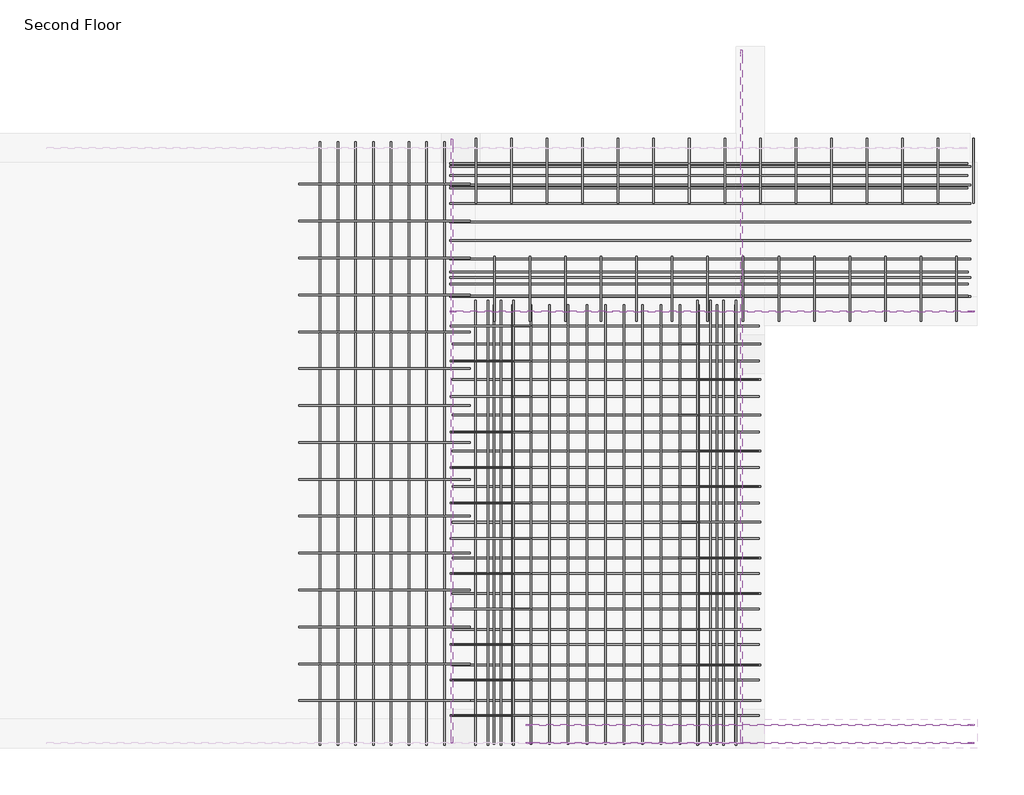
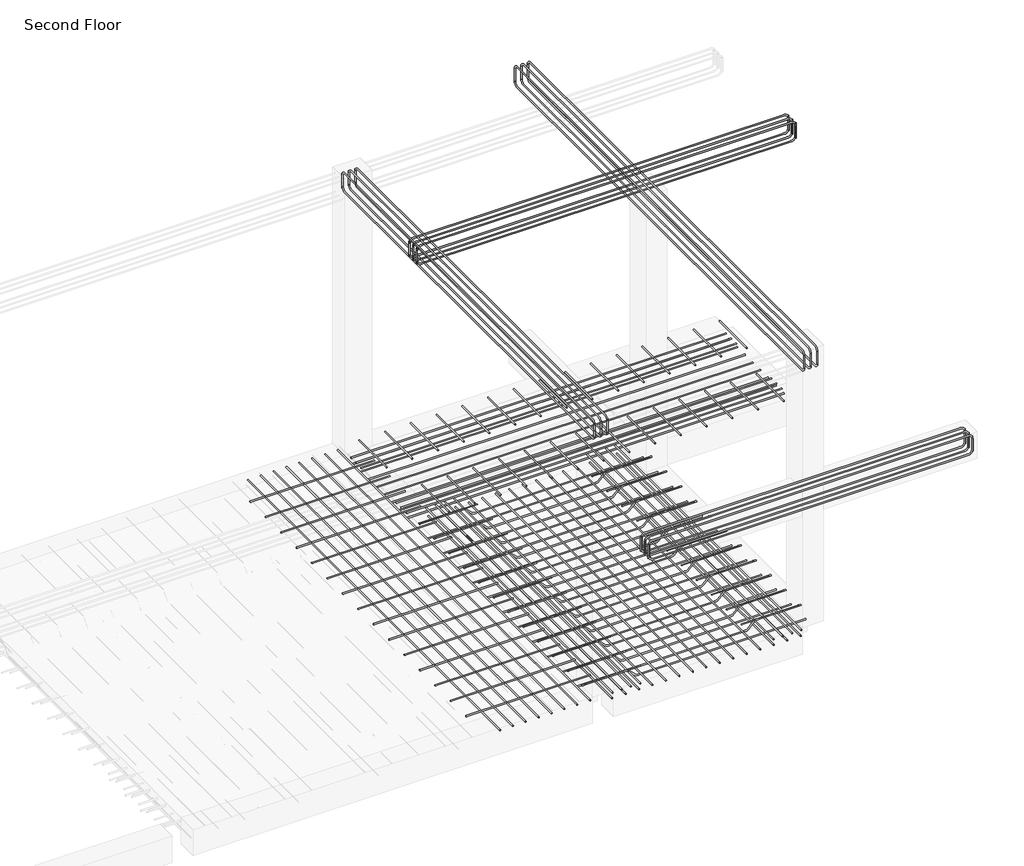
# One storey, part 4 of 4: 22 reinforcing bars.
"""IFC4 building model written with IfcOpenShell, lengths in millimetres."""

from ifc_helpers import new_model, si_unit, point, frame, origin, place, context, project, spatial, polyline, circle_curve, trimmed, segment, composite_curve, source, transform, mapped, element, save
from ifc_brep_helpers import swept_disk

model = new_model("IFC4")

# Units and contexts
model_context = context("Model", 3, world=origin())
ifc_project = project(units=[si_unit("LENGTHUNIT", "METRE", prefix="MILLI")], contexts=[model_context])

# Site, building, storey
site = spatial("IfcSite", under=ifc_project)
building = spatial("IfcBuilding", under=site)
storey = spatial("IfcBuildingStorey", under=building, Name="Second Floor", Elevation=6400.8)

# Reinforcing bars
placement = place(None, origin())
reinforcing_bar_shape = source(origin(), model_context, "Body", "SolidModel", [
    swept_disk(composite_curve([segment(polyline([(1701.2387526, 5017.2334631, 9363.3494949), (1701.2387526, 5017.2334631, 9511.3494949)]), True, "CONTINUOUS"), segment(trimmed(circle_curve(frame((1701.2387526, 4971.2334631, 9511.3494949), z_axis=(1.0, 0.0, 0.0), x_axis=(0.0, 46.0, 0.0)), 46.0), [point((1701.2387526, 5017.2334631, 9511.3494949))], [point((1701.2387526, 4971.2334631, 9557.3494949))], True, "CARTESIAN"), True, "CONTINUOUS"), segment(polyline([(1701.2387526, 4971.2334631, 9557.3494949), (1701.2387526, 278.4334631, 9557.3494949)]), True, "CONTINUOUS"), segment(trimmed(circle_curve(frame((1701.2387526, 278.4334631, 9511.3494949), z_axis=(1.0, 0.0, 0.0), x_axis=(0.0, 0.0, 46.0)), 46.0), [point((1701.2387526, 278.4334631, 9557.3494949))], [point((1701.2387526, 232.4334631, 9511.3494949))], True, "CARTESIAN"), True, "CONTINUOUS"), segment(polyline([(1701.2387526, 232.4334631, 9511.3494949), (1701.2387526, 232.4334631, 9363.3494949)]), True, "CONTINUOUS")], self_intersect=False), 6.0),
])
element("IfcReinforcingBar", 1, at=placement, inside=storey, context=model_context, shape_type="MappedRepresentation", body=[
    mapped(reinforcing_bar_shape, transform((0.0, 0.0, 0.0), x_axis=(1.0, 0.0, 0.0), y_axis=(0.0, 1.0, 0.0), z_axis=(0.0, 0.0, 1.0))),
    mapped(reinforcing_bar_shape, transform((70.4494949, 0.0, 0.0), x_axis=(1.0, 0.0, 0.0), y_axis=(0.0, 1.0, 0.0), z_axis=(0.0, 0.0, 1.0))),
    mapped(reinforcing_bar_shape, transform((140.8989899, 0.0, 0.0), x_axis=(1.0, 0.0, 0.0), y_axis=(0.0, 1.0, 0.0), z_axis=(0.0, 0.0, 1.0))),
])
reinforcing_bar_2_shape = source(origin(), model_context, "Body", "SolidModel", [
    swept_disk(composite_curve([segment(polyline([(1701.2387526, 5017.2334631, 9534.2505051), (1701.2387526, 5017.2334631, 9386.2505051)]), True, "CONTINUOUS"), segment(trimmed(circle_curve(frame((1701.2387526, 4971.2334631, 9386.2505051), z_axis=(-1.0, 0.0, 0.0), x_axis=(0.0, 46.0, 0.0)), 46.0), [point((1701.2387526, 5017.2334631, 9386.2505051))], [point((1701.2387526, 4971.2334631, 9340.2505051))], True, "CARTESIAN"), True, "CONTINUOUS"), segment(polyline([(1701.2387526, 4971.2334631, 9340.2505051), (1701.2387526, 278.4334631, 9340.2505051)]), True, "CONTINUOUS"), segment(trimmed(circle_curve(frame((1701.2387526, 278.4334631, 9386.2505051), z_axis=(-1.0, 0.0, 0.0), x_axis=(0.0, 0.0, -46.0)), 46.0), [point((1701.2387526, 278.4334631, 9340.2505051))], [point((1701.2387526, 232.4334631, 9386.2505051))], True, "CARTESIAN"), True, "CONTINUOUS"), segment(polyline([(1701.2387526, 232.4334631, 9386.2505051), (1701.2387526, 232.4334631, 9534.2505051)]), True, "CONTINUOUS")], self_intersect=False), 6.0),
])
element("IfcReinforcingBar", 2, at=placement, inside=storey, context=model_context, shape_type="MappedRepresentation", body=[
    mapped(reinforcing_bar_2_shape, transform((0.0, 0.0, 0.0), x_axis=(1.0, 0.0, 0.0), y_axis=(0.0, 1.0, 0.0), z_axis=(0.0, 0.0, 1.0))),
    mapped(reinforcing_bar_2_shape, transform((70.4494949, 0.0, 0.0), x_axis=(1.0, 0.0, 0.0), y_axis=(0.0, 1.0, 0.0), z_axis=(0.0, 0.0, 1.0))),
    mapped(reinforcing_bar_2_shape, transform((140.8989899, 0.0, 0.0), x_axis=(1.0, 0.0, 0.0), y_axis=(0.0, 1.0, 0.0), z_axis=(0.0, 0.0, 1.0))),
])
reinforcing_bar_3_shape = source(origin(), model_context, "Body", "SolidModel", [
    swept_disk(composite_curve([segment(polyline([(3999.1887526, 5724.7334631, 9364.0994949), (3999.1887526, 5724.7334631, 9512.0994949)]), True, "CONTINUOUS"), segment(trimmed(circle_curve(frame((3999.1887526, 5678.7334631, 9512.0994949), z_axis=(1.0, 0.0, 0.0), x_axis=(0.0, 46.0, 0.0)), 46.0), [point((3999.1887526, 5724.7334631, 9512.0994949))], [point((3999.1887526, 5678.7334631, 9558.0994949))], True, "CARTESIAN"), True, "CONTINUOUS"), segment(polyline([(3999.1887526, 5678.7334631, 9558.0994949), (3999.1887526, 278.4334631, 9558.0994949)]), True, "CONTINUOUS"), segment(trimmed(circle_curve(frame((3999.1887526, 278.4334631, 9512.0994949), z_axis=(1.0, 0.0, 0.0), x_axis=(0.0, 0.0, 46.0)), 46.0), [point((3999.1887526, 278.4334631, 9558.0994949))], [point((3999.1887526, 232.4334631, 9512.0994949))], True, "CARTESIAN"), True, "CONTINUOUS"), segment(polyline([(3999.1887526, 232.4334631, 9512.0994949), (3999.1887526, 232.4334631, 9364.0994949)]), True, "CONTINUOUS")], self_intersect=False), 6.0),
])
element("IfcReinforcingBar", 3, at=placement, inside=storey, context=model_context, shape_type="MappedRepresentation", body=[
    mapped(reinforcing_bar_3_shape, transform((0.0, 0.0, 0.0), x_axis=(1.0, 0.0, 0.0), y_axis=(0.0, 1.0, 0.0), z_axis=(0.0, 0.0, 1.0))),
    mapped(reinforcing_bar_3_shape, transform((71.1994949, 0.0, 0.0), x_axis=(1.0, 0.0, 0.0), y_axis=(0.0, 1.0, 0.0), z_axis=(0.0, 0.0, 1.0))),
    mapped(reinforcing_bar_3_shape, transform((142.3989899, 0.0, 0.0), x_axis=(1.0, 0.0, 0.0), y_axis=(0.0, 1.0, 0.0), z_axis=(0.0, 0.0, 1.0))),
])
reinforcing_bar_4_shape = source(origin(), model_context, "Body", "SolidModel", [
    swept_disk(composite_curve([segment(polyline([(3999.1887526, 5724.7334631, 9518.5005051), (3999.1887526, 5724.7334631, 9370.5005051)]), True, "CONTINUOUS"), segment(trimmed(circle_curve(frame((3999.1887526, 5678.7334631, 9370.5005051), z_axis=(-1.0, 0.0, 0.0), x_axis=(0.0, 46.0, 0.0)), 46.0), [point((3999.1887526, 5724.7334631, 9370.5005051))], [point((3999.1887526, 5678.7334631, 9324.5005051))], True, "CARTESIAN"), True, "CONTINUOUS"), segment(polyline([(3999.1887526, 5678.7334631, 9324.5005051), (3999.1887526, 278.4334631, 9324.5005051)]), True, "CONTINUOUS"), segment(trimmed(circle_curve(frame((3999.1887526, 278.4334631, 9370.5005051), z_axis=(-1.0, 0.0, 0.0), x_axis=(0.0, 0.0, -46.0)), 46.0), [point((3999.1887526, 278.4334631, 9324.5005051))], [point((3999.1887526, 232.4334631, 9370.5005051))], True, "CARTESIAN"), True, "CONTINUOUS"), segment(polyline([(3999.1887526, 232.4334631, 9370.5005051), (3999.1887526, 232.4334631, 9518.5005051)]), True, "CONTINUOUS")], self_intersect=False), 6.0),
])
element("IfcReinforcingBar", 4, at=placement, inside=storey, context=model_context, shape_type="MappedRepresentation", body=[
    mapped(reinforcing_bar_4_shape, transform((0.0, 0.0, 0.0), x_axis=(1.0, 0.0, 0.0), y_axis=(0.0, 1.0, 0.0), z_axis=(0.0, 0.0, 1.0))),
    mapped(reinforcing_bar_4_shape, transform((71.1994949, 0.0, 0.0), x_axis=(1.0, 0.0, 0.0), y_axis=(0.0, 1.0, 0.0), z_axis=(0.0, 0.0, 1.0))),
    mapped(reinforcing_bar_4_shape, transform((142.3989899, 0.0, 0.0), x_axis=(1.0, 0.0, 0.0), y_axis=(0.0, 1.0, 0.0), z_axis=(0.0, 0.0, 1.0))),
])
reinforcing_bar_5_shape = source(origin(), model_context, "Body", "SolidModel", [
    swept_disk(composite_curve([segment(polyline([(5841.2691711, 3584.0814555, 9362.3520076), (5841.2691711, 3584.0814555, 9510.3520076)]), True, "CONTINUOUS"), segment(trimmed(circle_curve(frame((5795.2691711, 3584.0814555, 9510.3520076), z_axis=(0.0, -1.0, 0.0), x_axis=(46.0, 0.0, 0.0)), 46.0), [point((5841.2691711, 3584.0814555, 9510.3520076))], [point((5795.2691711, 3584.0814555, 9556.3520076))], True, "CARTESIAN"), True, "CONTINUOUS"), segment(polyline([(5795.2691711, 3584.0814555, 9556.3520076), (1734.3882476, 3584.0814555, 9556.3520076)]), True, "CONTINUOUS"), segment(trimmed(circle_curve(frame((1734.3882476, 3584.0814555, 9510.3520076), z_axis=(0.0, -1.0, 0.0), x_axis=(0.0, 0.0, 46.0)), 46.0), [point((1734.3882476, 3584.0814555, 9556.3520076))], [point((1688.3882476, 3584.0814555, 9510.3520076))], True, "CARTESIAN"), True, "CONTINUOUS"), segment(polyline([(1688.3882476, 3584.0814555, 9510.3520076), (1688.3882476, 3584.0814555, 9362.3520076)]), True, "CONTINUOUS")], self_intersect=False), 6.0),
])
element("IfcReinforcingBar", 5, at=placement, inside=storey, context=model_context, shape_type="MappedRepresentation", body=[
    mapped(reinforcing_bar_5_shape, transform((0.0, 0.0, 0.0), x_axis=(1.0, 0.0, 0.0), y_axis=(0.0, 1.0, 0.0), z_axis=(0.0, 0.0, 1.0))),
    mapped(reinforcing_bar_5_shape, transform((0.0, 69.4520076, 0.0), x_axis=(1.0, 0.0, 0.0), y_axis=(0.0, 1.0, 0.0), z_axis=(0.0, 0.0, 1.0))),
    mapped(reinforcing_bar_5_shape, transform((0.0, 138.9040151, 0.0), x_axis=(1.0, 0.0, 0.0), y_axis=(0.0, 1.0, 0.0), z_axis=(0.0, 0.0, 1.0))),
])
reinforcing_bar_6_shape = source(origin(), model_context, "Body", "SolidModel", [
    swept_disk(composite_curve([segment(polyline([(5840.2625116, 3584.0814555, 9535.2479924), (5840.2625116, 3584.0814555, 9387.2479924)]), True, "CONTINUOUS"), segment(trimmed(circle_curve(frame((5794.2625116, 3584.0814555, 9387.2479924), z_axis=(0.0, 1.0, 0.0), x_axis=(46.0, 0.0, 0.0)), 46.0), [point((5840.2625116, 3584.0814555, 9387.2479924))], [point((5794.2625116, 3584.0814555, 9341.2479924))], True, "CARTESIAN"), True, "CONTINUOUS"), segment(polyline([(5794.2625116, 3584.0814555, 9341.2479924), (1734.3882476, 3584.0814555, 9341.2479924)]), True, "CONTINUOUS"), segment(trimmed(circle_curve(frame((1734.3882476, 3584.0814555, 9387.2479924), z_axis=(0.0, 1.0, 0.0), x_axis=(0.0, 0.0, -46.0)), 46.0), [point((1734.3882476, 3584.0814555, 9341.2479924))], [point((1688.3882476, 3584.0814555, 9387.2479924))], True, "CARTESIAN"), True, "CONTINUOUS"), segment(polyline([(1688.3882476, 3584.0814555, 9387.2479924), (1688.3882476, 3584.0814555, 9535.2479924)]), True, "CONTINUOUS")], self_intersect=False), 6.0),
])
element("IfcReinforcingBar", 6, at=placement, inside=storey, context=model_context, shape_type="MappedRepresentation", body=[
    mapped(reinforcing_bar_6_shape, transform((0.0, 0.0, 0.0), x_axis=(1.0, 0.0, 0.0), y_axis=(0.0, 1.0, 0.0), z_axis=(0.0, 0.0, 1.0))),
    mapped(reinforcing_bar_6_shape, transform((0.0, 69.4520076, 0.0), x_axis=(1.0, 0.0, 0.0), y_axis=(0.0, 1.0, 0.0), z_axis=(0.0, 0.0, 1.0))),
    mapped(reinforcing_bar_6_shape, transform((0.0, 138.9040151, 0.0), x_axis=(1.0, 0.0, 0.0), y_axis=(0.0, 1.0, 0.0), z_axis=(0.0, 0.0, 1.0))),
])
reinforcing_bar_7_shape = source(origin(), model_context, "Body", "SolidModel", [
    swept_disk(composite_curve([segment(polyline([(5841.2691711, 229.5339681, 7763.8994949), (5841.2691711, 229.5339681, 7911.8994949)]), True, "CONTINUOUS"), segment(trimmed(circle_curve(frame((5795.2691711, 229.5339681, 7911.8994949), z_axis=(0.0, -1.0, 0.0), x_axis=(46.0, 0.0, 0.0)), 46.0), [point((5841.2691711, 229.5339681, 7911.8994949))], [point((5795.2691711, 229.5339681, 7957.8994949))], True, "CARTESIAN"), True, "CONTINUOUS"), segment(polyline([(5795.2691711, 229.5339681, 7957.8994949), (2337.5636354, 229.5339681, 7957.8994949)]), True, "CONTINUOUS"), segment(trimmed(circle_curve(frame((2337.5636354, 229.5339681, 7911.8994949), z_axis=(0.0, -1.0, 0.0), x_axis=(0.0, 0.0, 46.0)), 46.0), [point((2337.5636354, 229.5339681, 7957.8994949))], [point((2291.5636354, 229.5339681, 7911.8994949))], True, "CARTESIAN"), True, "CONTINUOUS"), segment(polyline([(2291.5636354, 229.5339681, 7911.8994949), (2291.5636354, 229.5339681, 7763.8994949)]), True, "CONTINUOUS")], self_intersect=False), 6.0),
])
element("IfcReinforcingBar", 7, at=placement, inside=storey, context=model_context, shape_type="MappedRepresentation", body=[
    mapped(reinforcing_bar_7_shape, transform((0.0, 0.0, 0.0), x_axis=(1.0, 0.0, 0.0), y_axis=(0.0, 1.0, 0.0), z_axis=(0.0, 0.0, 1.0))),
    mapped(reinforcing_bar_7_shape, transform((0.0, 71.1994949, 0.0), x_axis=(1.0, 0.0, 0.0), y_axis=(0.0, 1.0, 0.0), z_axis=(0.0, 0.0, 1.0))),
    mapped(reinforcing_bar_7_shape, transform((0.0, 142.3989899, 0.0), x_axis=(1.0, 0.0, 0.0), y_axis=(0.0, 1.0, 0.0), z_axis=(0.0, 0.0, 1.0))),
])
reinforcing_bar_8_shape = source(origin(), model_context, "Body", "SolidModel", [
    swept_disk(composite_curve([segment(polyline([(5840.2625116, 229.5339681, 7933.3005051), (5840.2625116, 229.5339681, 7785.3005051)]), True, "CONTINUOUS"), segment(trimmed(circle_curve(frame((5794.2625116, 229.5339681, 7785.3005051), z_axis=(0.0, 1.0, 0.0), x_axis=(46.0, 0.0, 0.0)), 46.0), [point((5840.2625116, 229.5339681, 7785.3005051))], [point((5794.2625116, 229.5339681, 7739.3005051))], True, "CARTESIAN"), True, "CONTINUOUS"), segment(polyline([(5794.2625116, 229.5339681, 7739.3005051), (2341.190873, 229.5339681, 7739.3005051)]), True, "CONTINUOUS"), segment(trimmed(circle_curve(frame((2341.190873, 229.5339681, 7785.3005051), z_axis=(0.0, 1.0, 0.0), x_axis=(0.0, 0.0, -46.0)), 46.0), [point((2341.190873, 229.5339681, 7739.3005051))], [point((2295.190873, 229.5339681, 7785.3005051))], True, "CARTESIAN"), True, "CONTINUOUS"), segment(polyline([(2295.190873, 229.5339681, 7785.3005051), (2295.190873, 229.5339681, 7933.3005051)]), True, "CONTINUOUS")], self_intersect=False), 6.0),
])
element("IfcReinforcingBar", 8, at=placement, inside=storey, context=model_context, shape_type="MappedRepresentation", body=[
    mapped(reinforcing_bar_8_shape, transform((0.0, 0.0, 0.0), x_axis=(1.0, 0.0, 0.0), y_axis=(0.0, 1.0, 0.0), z_axis=(0.0, 0.0, 1.0))),
    mapped(reinforcing_bar_8_shape, transform((0.0, 71.1994949, 0.0), x_axis=(1.0, 0.0, 0.0), y_axis=(0.0, 1.0, 0.0), z_axis=(0.0, 0.0, 1.0))),
    mapped(reinforcing_bar_8_shape, transform((0.0, 142.3989899, 0.0), x_axis=(1.0, 0.0, 0.0), y_axis=(0.0, 1.0, 0.0), z_axis=(0.0, 0.0, 1.0))),
])
reinforcing_bar_9_shape = source(origin(), model_context, "Body", "SolidModel", [
    swept_disk(composite_curve([segment(polyline([(1688.7874305, 3539.2334631, 6369.8), (2168.5956769, 3539.2334631, 6369.8)]), True, "CONTINUOUS"), segment(trimmed(circle_curve(frame((2168.5956769, 3539.2334631, 6323.8), z_axis=(0.0, 1.0, 0.0), x_axis=(0.0, 0.0, 46.0)), 46.0), [point((2168.5956769, 3539.2334631, 6369.8))], [point((2201.1225888, 3539.2334631, 6356.3269119))], True, "CARTESIAN"), True, "CONTINUOUS"), segment(polyline([(2201.1225888, 3539.2334631, 6356.3269119), (2264.5764127, 3539.2334631, 6292.8730881)]), True, "CONTINUOUS"), segment(trimmed(circle_curve(frame((2297.1033246, 3539.2334631, 6325.4), z_axis=(0.0, -1.0, 0.0), x_axis=(-32.52691189999996, 0.0, -32.526911899999504)), 46.0), [point((2264.5764127, 3539.2334631, 6292.8730881))], [point((2297.1033246, 3539.2334631, 6279.4))], True, "CARTESIAN"), True, "CONTINUOUS"), segment(polyline([(2297.1033246, 3539.2334631, 6279.4), (4139.8402551, 3539.2334631, 6279.4)]), True, "CONTINUOUS")], self_intersect=False), 6.0),
])
element("IfcReinforcingBar", 9, at=placement, inside=storey, context=model_context, shape_type="MappedRepresentation", body=[
    mapped(reinforcing_bar_9_shape, transform((0.0, 0.0, 0.0), x_axis=(1.0, 0.0, 0.0), y_axis=(0.0, 1.0, 0.0), z_axis=(0.0, 0.0, 1.0))),
    mapped(reinforcing_bar_9_shape, transform((0.0, -281.0909091, 0.0), x_axis=(1.0, 0.0, 0.0), y_axis=(0.0, 1.0, 0.0), z_axis=(0.0, 0.0, 1.0))),
    mapped(reinforcing_bar_9_shape, transform((0.0, -562.1818182, 0.0), x_axis=(1.0, 0.0, 0.0), y_axis=(0.0, 1.0, 0.0), z_axis=(0.0, 0.0, 1.0))),
    mapped(reinforcing_bar_9_shape, transform((0.0, -843.2727273, 0.0), x_axis=(1.0, 0.0, 0.0), y_axis=(0.0, 1.0, 0.0), z_axis=(0.0, 0.0, 1.0))),
    mapped(reinforcing_bar_9_shape, transform((0.0, -1124.3636364, 0.0), x_axis=(1.0, 0.0, 0.0), y_axis=(0.0, 1.0, 0.0), z_axis=(0.0, 0.0, 1.0))),
    mapped(reinforcing_bar_9_shape, transform((0.0, -1405.4545455, 0.0), x_axis=(1.0, 0.0, 0.0), y_axis=(0.0, 1.0, 0.0), z_axis=(0.0, 0.0, 1.0))),
    mapped(reinforcing_bar_9_shape, transform((0.0, -1686.5454545, 0.0), x_axis=(1.0, 0.0, 0.0), y_axis=(0.0, 1.0, 0.0), z_axis=(0.0, 0.0, 1.0))),
    mapped(reinforcing_bar_9_shape, transform((0.0, -1967.6363636, 0.0), x_axis=(1.0, 0.0, 0.0), y_axis=(0.0, 1.0, 0.0), z_axis=(0.0, 0.0, 1.0))),
    mapped(reinforcing_bar_9_shape, transform((0.0, -2248.7272727, 0.0), x_axis=(1.0, 0.0, 0.0), y_axis=(0.0, 1.0, 0.0), z_axis=(0.0, 0.0, 1.0))),
    mapped(reinforcing_bar_9_shape, transform((0.0, -2529.8181818, 0.0), x_axis=(1.0, 0.0, 0.0), y_axis=(0.0, 1.0, 0.0), z_axis=(0.0, 0.0, 1.0))),
    mapped(reinforcing_bar_9_shape, transform((0.0, -2810.9090909, 0.0), x_axis=(1.0, 0.0, 0.0), y_axis=(0.0, 1.0, 0.0), z_axis=(0.0, 0.0, 1.0))),
    mapped(reinforcing_bar_9_shape, transform((0.0, -3092.0, 0.0), x_axis=(1.0, 0.0, 0.0), y_axis=(0.0, 1.0, 0.0), z_axis=(0.0, 0.0, 1.0))),
])
reinforcing_bar_10_shape = source(origin(), model_context, "Body", "SolidModel", [
    swept_disk(composite_curve([segment(polyline([(4153.2890646, 564.2307141, 6369.8), (3672.2951557, 564.2307141, 6369.8)]), True, "CONTINUOUS"), segment(trimmed(circle_curve(frame((3672.2951557, 564.2307141, 6323.8), z_axis=(0.0, -1.0, 0.0), x_axis=(0.0, 0.0, 46.0)), 46.0), [point((3672.2951557, 564.2307141, 6369.8))], [point((3639.7682438, 564.2307141, 6356.3269119))], True, "CARTESIAN"), True, "CONTINUOUS"), segment(polyline([(3639.7682438, 564.2307141, 6356.3269119), (3576.3144199, 564.2307141, 6292.8730881)]), True, "CONTINUOUS"), segment(trimmed(circle_curve(frame((3543.787508, 564.2307141, 6325.4), z_axis=(0.0, 1.0000000000000002, 0.0), x_axis=(32.52691189999996, 0.0, -32.526911899999504)), 46.0), [point((3576.3144199, 564.2307141, 6292.8730881))], [point((3543.787508, 564.2307141, 6279.4))], True, "CARTESIAN"), True, "CONTINUOUS"), segment(polyline([(3543.787508, 564.2307141, 6279.4), (1702.23624, 564.2307141, 6279.4)]), True, "CONTINUOUS")], self_intersect=False), 6.0),
])
element("IfcReinforcingBar", 10, at=placement, inside=storey, context=model_context, shape_type="MappedRepresentation", body=[
    mapped(reinforcing_bar_10_shape, transform((0.0, 0.0, 0.0), x_axis=(1.0, 0.0, 0.0), y_axis=(0.0, 1.0, 0.0), z_axis=(0.0, 0.0, 1.0))),
    mapped(reinforcing_bar_10_shape, transform((0.0, 283.1945647, 0.0), x_axis=(1.0, 0.0, 0.0), y_axis=(0.0, 1.0, 0.0), z_axis=(0.0, 0.0, 1.0))),
    mapped(reinforcing_bar_10_shape, transform((0.0, 566.3891295, 0.0), x_axis=(1.0, 0.0, 0.0), y_axis=(0.0, 1.0, 0.0), z_axis=(0.0, 0.0, 1.0))),
    mapped(reinforcing_bar_10_shape, transform((0.0, 849.5836942, 0.0), x_axis=(1.0, 0.0, 0.0), y_axis=(0.0, 1.0, 0.0), z_axis=(0.0, 0.0, 1.0))),
    mapped(reinforcing_bar_10_shape, transform((0.0, 1132.778259, 0.0), x_axis=(1.0, 0.0, 0.0), y_axis=(0.0, 1.0, 0.0), z_axis=(0.0, 0.0, 1.0))),
    mapped(reinforcing_bar_10_shape, transform((0.0, 1415.9728237, 0.0), x_axis=(1.0, 0.0, 0.0), y_axis=(0.0, 1.0, 0.0), z_axis=(0.0, 0.0, 1.0))),
    mapped(reinforcing_bar_10_shape, transform((0.0, 1699.1673885, 0.0), x_axis=(1.0, 0.0, 0.0), y_axis=(0.0, 1.0, 0.0), z_axis=(0.0, 0.0, 1.0))),
    mapped(reinforcing_bar_10_shape, transform((0.0, 1982.3619532, 0.0), x_axis=(1.0, 0.0, 0.0), y_axis=(0.0, 1.0, 0.0), z_axis=(0.0, 0.0, 1.0))),
    mapped(reinforcing_bar_10_shape, transform((0.0, 2265.556518, 0.0), x_axis=(1.0, 0.0, 0.0), y_axis=(0.0, 1.0, 0.0), z_axis=(0.0, 0.0, 1.0))),
    mapped(reinforcing_bar_10_shape, transform((0.0, 2548.7510827, 0.0), x_axis=(1.0, 0.0, 0.0), y_axis=(0.0, 1.0, 0.0), z_axis=(0.0, 0.0, 1.0))),
    mapped(reinforcing_bar_10_shape, transform((0.0, 2831.9456475, 0.0), x_axis=(1.0, 0.0, 0.0), y_axis=(0.0, 1.0, 0.0), z_axis=(0.0, 0.0, 1.0))),
])
reinforcing_bar_11_shape = source(origin(), model_context, "Body", "SolidModel", [
    swept_disk(composite_curve([segment(polyline([(3650.7560505, 3742.8334631, 6359.5006995), (3650.7560505, 211.4334631, 6359.5006995)]), True, "CONTINUOUS")], self_intersect=False), 6.0),
])
element("IfcReinforcingBar", 11, at=placement, inside=storey, context=model_context, shape_type="MappedRepresentation", body=[
    mapped(reinforcing_bar_11_shape, transform((0.0, 0.0, 0.0), x_axis=(1.0, 0.0, 0.0), y_axis=(0.0, 1.0, 0.0), z_axis=(0.0, 0.0, 1.0))),
    mapped(reinforcing_bar_11_shape, transform((101.777399, 0.0, 0.0), x_axis=(1.0, 0.0, 0.0), y_axis=(0.0, 1.0, 0.0), z_axis=(0.0, 0.0, 1.0))),
    mapped(reinforcing_bar_11_shape, transform((203.554798, 0.0, 0.0), x_axis=(1.0, 0.0, 0.0), y_axis=(0.0, 1.0, 0.0), z_axis=(0.0, 0.0, 1.0))),
    mapped(reinforcing_bar_11_shape, transform((305.3321971, 0.0, 0.0), x_axis=(1.0, 0.0, 0.0), y_axis=(0.0, 1.0, 0.0), z_axis=(0.0, 0.0, 1.0))),
])
reinforcing_bar_12_shape = source(origin(), model_context, "Body", "SolidModel", [
    swept_disk(composite_curve([segment(polyline([(1697.8477074, 3539.2334631, 6371.8), (2325.3671503, 3539.2334631, 6371.8)]), True, "CONTINUOUS")], self_intersect=False), 4.0),
])
element("IfcReinforcingBar", 12, at=placement, inside=storey, context=model_context, shape_type="MappedRepresentation", body=[
    mapped(reinforcing_bar_12_shape, transform((0.0, 0.0, 0.0), x_axis=(1.0, 0.0, 0.0), y_axis=(0.0, 1.0, 0.0), z_axis=(0.0, 0.0, 1.0))),
    mapped(reinforcing_bar_12_shape, transform((0.0, -281.0909091, 0.0), x_axis=(1.0, 0.0, 0.0), y_axis=(0.0, 1.0, 0.0), z_axis=(0.0, 0.0, 1.0))),
    mapped(reinforcing_bar_12_shape, transform((0.0, -562.1818182, 0.0), x_axis=(1.0, 0.0, 0.0), y_axis=(0.0, 1.0, 0.0), z_axis=(0.0, 0.0, 1.0))),
    mapped(reinforcing_bar_12_shape, transform((0.0, -843.2727273, 0.0), x_axis=(1.0, 0.0, 0.0), y_axis=(0.0, 1.0, 0.0), z_axis=(0.0, 0.0, 1.0))),
    mapped(reinforcing_bar_12_shape, transform((0.0, -1124.3636364, 0.0), x_axis=(1.0, 0.0, 0.0), y_axis=(0.0, 1.0, 0.0), z_axis=(0.0, 0.0, 1.0))),
    mapped(reinforcing_bar_12_shape, transform((0.0, -1405.4545455, 0.0), x_axis=(1.0, 0.0, 0.0), y_axis=(0.0, 1.0, 0.0), z_axis=(0.0, 0.0, 1.0))),
    mapped(reinforcing_bar_12_shape, transform((0.0, -1686.5454545, 0.0), x_axis=(1.0, 0.0, 0.0), y_axis=(0.0, 1.0, 0.0), z_axis=(0.0, 0.0, 1.0))),
    mapped(reinforcing_bar_12_shape, transform((0.0, -1967.6363636, 0.0), x_axis=(1.0, 0.0, 0.0), y_axis=(0.0, 1.0, 0.0), z_axis=(0.0, 0.0, 1.0))),
    mapped(reinforcing_bar_12_shape, transform((0.0, -2248.7272727, 0.0), x_axis=(1.0, 0.0, 0.0), y_axis=(0.0, 1.0, 0.0), z_axis=(0.0, 0.0, 1.0))),
    mapped(reinforcing_bar_12_shape, transform((0.0, -2529.8181818, 0.0), x_axis=(1.0, 0.0, 0.0), y_axis=(0.0, 1.0, 0.0), z_axis=(0.0, 0.0, 1.0))),
    mapped(reinforcing_bar_12_shape, transform((0.0, -2810.9090909, 0.0), x_axis=(1.0, 0.0, 0.0), y_axis=(0.0, 1.0, 0.0), z_axis=(0.0, 0.0, 1.0))),
    mapped(reinforcing_bar_12_shape, transform((0.0, -3092.0, 0.0), x_axis=(1.0, 0.0, 0.0), y_axis=(0.0, 1.0, 0.0), z_axis=(0.0, 0.0, 1.0))),
])
reinforcing_bar_13_shape = source(origin(), model_context, "Body", "SolidModel", [
    swept_disk(composite_curve([segment(polyline([(4130.5876361, 3396.1763616, 6371.8), (3500.3340616, 3396.1763616, 6371.8)]), True, "CONTINUOUS")], self_intersect=False), 4.0),
])
element("IfcReinforcingBar", 13, at=placement, inside=storey, context=model_context, shape_type="MappedRepresentation", body=[
    mapped(reinforcing_bar_13_shape, transform((0.0, 0.0, 0.0), x_axis=(1.0, 0.0, 0.0), y_axis=(0.0, 1.0, 0.0), z_axis=(0.0, 0.0, 1.0))),
    mapped(reinforcing_bar_13_shape, transform((0.0, -283.1945647, 0.0), x_axis=(1.0, 0.0, 0.0), y_axis=(0.0, 1.0, 0.0), z_axis=(0.0, 0.0, 1.0))),
    mapped(reinforcing_bar_13_shape, transform((0.0, -566.3891295, 0.0), x_axis=(1.0, 0.0, 0.0), y_axis=(0.0, 1.0, 0.0), z_axis=(0.0, 0.0, 1.0))),
    mapped(reinforcing_bar_13_shape, transform((0.0, -849.5836942, 0.0), x_axis=(1.0, 0.0, 0.0), y_axis=(0.0, 1.0, 0.0), z_axis=(0.0, 0.0, 1.0))),
    mapped(reinforcing_bar_13_shape, transform((0.0, -1132.778259, 0.0), x_axis=(1.0, 0.0, 0.0), y_axis=(0.0, 1.0, 0.0), z_axis=(0.0, 0.0, 1.0))),
    mapped(reinforcing_bar_13_shape, transform((0.0, -1415.9728237, 0.0), x_axis=(1.0, 0.0, 0.0), y_axis=(0.0, 1.0, 0.0), z_axis=(0.0, 0.0, 1.0))),
    mapped(reinforcing_bar_13_shape, transform((0.0, -1699.1673885, 0.0), x_axis=(1.0, 0.0, 0.0), y_axis=(0.0, 1.0, 0.0), z_axis=(0.0, 0.0, 1.0))),
    mapped(reinforcing_bar_13_shape, transform((0.0, -1982.3619532, 0.0), x_axis=(1.0, 0.0, 0.0), y_axis=(0.0, 1.0, 0.0), z_axis=(0.0, 0.0, 1.0))),
    mapped(reinforcing_bar_13_shape, transform((0.0, -2265.556518, 0.0), x_axis=(1.0, 0.0, 0.0), y_axis=(0.0, 1.0, 0.0), z_axis=(0.0, 0.0, 1.0))),
    mapped(reinforcing_bar_13_shape, transform((0.0, -2548.7510827, 0.0), x_axis=(1.0, 0.0, 0.0), y_axis=(0.0, 1.0, 0.0), z_axis=(0.0, 0.0, 1.0))),
    mapped(reinforcing_bar_13_shape, transform((0.0, -2831.9456475, 0.0), x_axis=(1.0, 0.0, 0.0), y_axis=(0.0, 1.0, 0.0), z_axis=(0.0, 0.0, 1.0))),
])
reinforcing_bar_14_shape = source(origin(), model_context, "Body", "SolidModel", [
    swept_disk(composite_curve([segment(polyline([(3952.0882476, 218.9117605, 6287.9387401), (3952.0882476, 3706.6679133, 6287.9387401)]), True, "CONTINUOUS")], self_intersect=False), 6.0),
])
element("IfcReinforcingBar", 14, at=placement, inside=storey, context=model_context, shape_type="MappedRepresentation", body=[
    mapped(reinforcing_bar_14_shape, transform((0.0, 0.0, 0.0), x_axis=(1.0, 0.0, 0.0), y_axis=(0.0, 1.0, 0.0), z_axis=(0.0, 0.0, 1.0))),
    mapped(reinforcing_bar_14_shape, transform((-147.5785714, 0.0, 0.0), x_axis=(1.0, 0.0, 0.0), y_axis=(0.0, 1.0, 0.0), z_axis=(0.0, 0.0, 1.0))),
    mapped(reinforcing_bar_14_shape, transform((-295.1571429, 0.0, 0.0), x_axis=(1.0, 0.0, 0.0), y_axis=(0.0, 1.0, 0.0), z_axis=(0.0, 0.0, 1.0))),
    mapped(reinforcing_bar_14_shape, transform((-442.7357143, 0.0, 0.0), x_axis=(1.0, 0.0, 0.0), y_axis=(0.0, 1.0, 0.0), z_axis=(0.0, 0.0, 1.0))),
    mapped(reinforcing_bar_14_shape, transform((-590.3142857, 0.0, 0.0), x_axis=(1.0, 0.0, 0.0), y_axis=(0.0, 1.0, 0.0), z_axis=(0.0, 0.0, 1.0))),
    mapped(reinforcing_bar_14_shape, transform((-737.8928571, 0.0, 0.0), x_axis=(1.0, 0.0, 0.0), y_axis=(0.0, 1.0, 0.0), z_axis=(0.0, 0.0, 1.0))),
    mapped(reinforcing_bar_14_shape, transform((-885.4714286, 0.0, 0.0), x_axis=(1.0, 0.0, 0.0), y_axis=(0.0, 1.0, 0.0), z_axis=(0.0, 0.0, 1.0))),
    mapped(reinforcing_bar_14_shape, transform((-1033.05, 0.0, 0.0), x_axis=(1.0, 0.0, 0.0), y_axis=(0.0, 1.0, 0.0), z_axis=(0.0, 0.0, 1.0))),
    mapped(reinforcing_bar_14_shape, transform((-1180.6285714, 0.0, 0.0), x_axis=(1.0, 0.0, 0.0), y_axis=(0.0, 1.0, 0.0), z_axis=(0.0, 0.0, 1.0))),
    mapped(reinforcing_bar_14_shape, transform((-1328.2071429, 0.0, 0.0), x_axis=(1.0, 0.0, 0.0), y_axis=(0.0, 1.0, 0.0), z_axis=(0.0, 0.0, 1.0))),
    mapped(reinforcing_bar_14_shape, transform((-1475.7857143, 0.0, 0.0), x_axis=(1.0, 0.0, 0.0), y_axis=(0.0, 1.0, 0.0), z_axis=(0.0, 0.0, 1.0))),
    mapped(reinforcing_bar_14_shape, transform((-1623.3642857, 0.0, 0.0), x_axis=(1.0, 0.0, 0.0), y_axis=(0.0, 1.0, 0.0), z_axis=(0.0, 0.0, 1.0))),
    mapped(reinforcing_bar_14_shape, transform((-1770.9428571, 0.0, 0.0), x_axis=(1.0, 0.0, 0.0), y_axis=(0.0, 1.0, 0.0), z_axis=(0.0, 0.0, 1.0))),
    mapped(reinforcing_bar_14_shape, transform((-1918.5214286, 0.0, 0.0), x_axis=(1.0, 0.0, 0.0), y_axis=(0.0, 1.0, 0.0), z_axis=(0.0, 0.0, 1.0))),
    mapped(reinforcing_bar_14_shape, transform((-2066.1, 0.0, 0.0), x_axis=(1.0, 0.0, 0.0), y_axis=(0.0, 1.0, 0.0), z_axis=(0.0, 0.0, 1.0))),
])
reinforcing_bar_15_shape = source(origin(), model_context, "Body", "SolidModel", [
    swept_disk(composite_curve([segment(polyline([(2190.1347821, 3742.8334631, 6359.5006995), (2190.1347821, 211.4334631, 6359.5006995)]), True, "CONTINUOUS")], self_intersect=False), 6.0),
])
element("IfcReinforcingBar", 15, at=placement, inside=storey, context=model_context, shape_type="MappedRepresentation", body=[
    mapped(reinforcing_bar_15_shape, transform((0.0, 0.0, 0.0), x_axis=(1.0, 0.0, 0.0), y_axis=(0.0, 1.0, 0.0), z_axis=(0.0, 0.0, 1.0))),
    mapped(reinforcing_bar_15_shape, transform((-101.3821782, 0.0, 0.0), x_axis=(1.0, 0.0, 0.0), y_axis=(0.0, 1.0, 0.0), z_axis=(0.0, 0.0, 1.0))),
    mapped(reinforcing_bar_15_shape, transform((-202.7643564, 0.0, 0.0), x_axis=(1.0, 0.0, 0.0), y_axis=(0.0, 1.0, 0.0), z_axis=(0.0, 0.0, 1.0))),
    mapped(reinforcing_bar_15_shape, transform((-304.1465345, 0.0, 0.0), x_axis=(1.0, 0.0, 0.0), y_axis=(0.0, 1.0, 0.0), z_axis=(0.0, 0.0, 1.0))),
])
reinforcing_bar_16_shape = source(origin(), model_context, "Body", "SolidModel", [
    swept_disk(composite_curve([segment(polyline([(654.4332967, 4999.0798317, 6354.8697281), (654.4332967, 211.4334631, 6354.8697281)]), True, "CONTINUOUS")], self_intersect=False), 6.0),
])
element("IfcReinforcingBar", 16, at=placement, inside=storey, context=model_context, shape_type="MappedRepresentation", body=[
    mapped(reinforcing_bar_16_shape, transform((0.0, 0.0, 0.0), x_axis=(1.0, 0.0, 0.0), y_axis=(0.0, 1.0, 0.0), z_axis=(0.0, 0.0, 1.0))),
    mapped(reinforcing_bar_16_shape, transform((140.8412233, 0.0, 0.0), x_axis=(1.0, 0.0, 0.0), y_axis=(0.0, 1.0, 0.0), z_axis=(0.0, 0.0, 1.0))),
    mapped(reinforcing_bar_16_shape, transform((281.6824466, 0.0, 0.0), x_axis=(1.0, 0.0, 0.0), y_axis=(0.0, 1.0, 0.0), z_axis=(0.0, 0.0, 1.0))),
    mapped(reinforcing_bar_16_shape, transform((422.5236699, 0.0, 0.0), x_axis=(1.0, 0.0, 0.0), y_axis=(0.0, 1.0, 0.0), z_axis=(0.0, 0.0, 1.0))),
    mapped(reinforcing_bar_16_shape, transform((563.3648932, 0.0, 0.0), x_axis=(1.0, 0.0, 0.0), y_axis=(0.0, 1.0, 0.0), z_axis=(0.0, 0.0, 1.0))),
    mapped(reinforcing_bar_16_shape, transform((704.2061164, 0.0, 0.0), x_axis=(1.0, 0.0, 0.0), y_axis=(0.0, 1.0, 0.0), z_axis=(0.0, 0.0, 1.0))),
    mapped(reinforcing_bar_16_shape, transform((845.0473397, 0.0, 0.0), x_axis=(1.0, 0.0, 0.0), y_axis=(0.0, 1.0, 0.0), z_axis=(0.0, 0.0, 1.0))),
    mapped(reinforcing_bar_16_shape, transform((985.888563, 0.0, 0.0), x_axis=(1.0, 0.0, 0.0), y_axis=(0.0, 1.0, 0.0), z_axis=(0.0, 0.0, 1.0))),
])
reinforcing_bar_17_shape = source(origin(), model_context, "Body", "SolidModel", [
    swept_disk(composite_curve([segment(polyline([(1844.9074635, 564.2307141, 6364.2017937), (483.2910842, 564.2307141, 6364.2017937)]), True, "CONTINUOUS")], self_intersect=False), 6.0),
])
element("IfcReinforcingBar", 17, at=placement, inside=storey, context=model_context, shape_type="MappedRepresentation", body=[
    mapped(reinforcing_bar_17_shape, transform((0.0, 0.0, 0.0), x_axis=(1.0, 0.0, 0.0), y_axis=(0.0, 1.0, 0.0), z_axis=(0.0, 0.0, 1.0))),
    mapped(reinforcing_bar_17_shape, transform((0.0, 292.7783831, 0.0), x_axis=(1.0, 0.0, 0.0), y_axis=(0.0, 1.0, 0.0), z_axis=(0.0, 0.0, 1.0))),
    mapped(reinforcing_bar_17_shape, transform((0.0, 585.5567661, 0.0), x_axis=(1.0, 0.0, 0.0), y_axis=(0.0, 1.0, 0.0), z_axis=(0.0, 0.0, 1.0))),
    mapped(reinforcing_bar_17_shape, transform((0.0, 878.3351492, 0.0), x_axis=(1.0, 0.0, 0.0), y_axis=(0.0, 1.0, 0.0), z_axis=(0.0, 0.0, 1.0))),
    mapped(reinforcing_bar_17_shape, transform((0.0, 1171.1135323, 0.0), x_axis=(1.0, 0.0, 0.0), y_axis=(0.0, 1.0, 0.0), z_axis=(0.0, 0.0, 1.0))),
    mapped(reinforcing_bar_17_shape, transform((0.0, 1463.8919154, 0.0), x_axis=(1.0, 0.0, 0.0), y_axis=(0.0, 1.0, 0.0), z_axis=(0.0, 0.0, 1.0))),
    mapped(reinforcing_bar_17_shape, transform((0.0, 1756.6702984, 0.0), x_axis=(1.0, 0.0, 0.0), y_axis=(0.0, 1.0, 0.0), z_axis=(0.0, 0.0, 1.0))),
    mapped(reinforcing_bar_17_shape, transform((0.0, 2049.4486815, 0.0), x_axis=(1.0, 0.0, 0.0), y_axis=(0.0, 1.0, 0.0), z_axis=(0.0, 0.0, 1.0))),
    mapped(reinforcing_bar_17_shape, transform((0.0, 2342.2270646, 0.0), x_axis=(1.0, 0.0, 0.0), y_axis=(0.0, 1.0, 0.0), z_axis=(0.0, 0.0, 1.0))),
    mapped(reinforcing_bar_17_shape, transform((0.0, 2635.0054477, 0.0), x_axis=(1.0, 0.0, 0.0), y_axis=(0.0, 1.0, 0.0), z_axis=(0.0, 0.0, 1.0))),
    mapped(reinforcing_bar_17_shape, transform((0.0, 2927.7838307, 0.0), x_axis=(1.0, 0.0, 0.0), y_axis=(0.0, 1.0, 0.0), z_axis=(0.0, 0.0, 1.0))),
    mapped(reinforcing_bar_17_shape, transform((0.0, 3220.5622138, 0.0), x_axis=(1.0, 0.0, 0.0), y_axis=(0.0, 1.0, 0.0), z_axis=(0.0, 0.0, 1.0))),
    mapped(reinforcing_bar_17_shape, transform((0.0, 3513.3405969, 0.0), x_axis=(1.0, 0.0, 0.0), y_axis=(0.0, 1.0, 0.0), z_axis=(0.0, 0.0, 1.0))),
    mapped(reinforcing_bar_17_shape, transform((0.0, 3806.11898, 0.0), x_axis=(1.0, 0.0, 0.0), y_axis=(0.0, 1.0, 0.0), z_axis=(0.0, 0.0, 1.0))),
    mapped(reinforcing_bar_17_shape, transform((0.0, 4098.897363, 0.0), x_axis=(1.0, 0.0, 0.0), y_axis=(0.0, 1.0, 0.0), z_axis=(0.0, 0.0, 1.0))),
])
reinforcing_bar_18_shape = source(origin(), model_context, "Body", "SolidModel", [
    swept_disk(composite_curve([segment(polyline([(5796.3354159, 4634.2611065, 6354.7212824), (1682.3882476, 4634.2611065, 6354.7212824)]), True, "CONTINUOUS")], self_intersect=False), 6.0),
])
element("IfcReinforcingBar", 18, at=placement, inside=storey, context=model_context, shape_type="MappedRepresentation", body=[
    mapped(reinforcing_bar_18_shape, transform((0.0, 0.0, 0.0), x_axis=(1.0, 0.0, 0.0), y_axis=(0.0, 1.0, 0.0), z_axis=(0.0, 0.0, 1.0))),
    mapped(reinforcing_bar_18_shape, transform((0.0, 96.3869435, 0.0), x_axis=(1.0, 0.0, 0.0), y_axis=(0.0, 1.0, 0.0), z_axis=(0.0, 0.0, 1.0))),
    mapped(reinforcing_bar_18_shape, transform((0.0, 192.773887, 0.0), x_axis=(1.0, 0.0, 0.0), y_axis=(0.0, 1.0, 0.0), z_axis=(0.0, 0.0, 1.0))),
])
reinforcing_bar_19_shape = source(origin(), model_context, "Body", "SolidModel", [
    swept_disk(composite_curve([segment(polyline([(5798.6824692, 3968.2058196, 6354.7212824), (1682.3882476, 3968.2058196, 6354.7212824)]), True, "CONTINUOUS")], self_intersect=False), 6.0),
])
element("IfcReinforcingBar", 19, at=placement, inside=storey, context=model_context, shape_type="MappedRepresentation", body=[
    mapped(reinforcing_bar_19_shape, transform((0.0, 0.0, 0.0), x_axis=(1.0, 0.0, 0.0), y_axis=(0.0, 1.0, 0.0), z_axis=(0.0, 0.0, 1.0))),
    mapped(reinforcing_bar_19_shape, transform((0.0, -96.3869435, 0.0), x_axis=(1.0, 0.0, 0.0), y_axis=(0.0, 1.0, 0.0), z_axis=(0.0, 0.0, 1.0))),
    mapped(reinforcing_bar_19_shape, transform((0.0, -192.773887, 0.0), x_axis=(1.0, 0.0, 0.0), y_axis=(0.0, 1.0, 0.0), z_axis=(0.0, 0.0, 1.0))),
])
reinforcing_bar_20_shape = source(origin(), model_context, "Body", "SolidModel", [
    swept_disk(composite_curve([segment(polyline([(5840.6882476, 5026.8576948, 6362.9336733), (5840.6882476, 4511.8136411, 6362.9336733)]), True, "CONTINUOUS")], self_intersect=False), 6.0),
])
element("IfcReinforcingBar", 20, at=placement, inside=storey, context=model_context, shape_type="MappedRepresentation", body=[
    mapped(reinforcing_bar_20_shape, transform((0.0, 0.0, 0.0), x_axis=(1.0, 0.0, 0.0), y_axis=(0.0, 1.0, 0.0), z_axis=(0.0, 0.0, 1.0))),
    mapped(reinforcing_bar_20_shape, transform((-282.05, 0.0, 0.0), x_axis=(1.0, 0.0, 0.0), y_axis=(0.0, 1.0, 0.0), z_axis=(0.0, 0.0, 1.0))),
    mapped(reinforcing_bar_20_shape, transform((-564.1, 0.0, 0.0), x_axis=(1.0, 0.0, 0.0), y_axis=(0.0, 1.0, 0.0), z_axis=(0.0, 0.0, 1.0))),
    mapped(reinforcing_bar_20_shape, transform((-846.15, 0.0, 0.0), x_axis=(1.0, 0.0, 0.0), y_axis=(0.0, 1.0, 0.0), z_axis=(0.0, 0.0, 1.0))),
    mapped(reinforcing_bar_20_shape, transform((-1128.2, 0.0, 0.0), x_axis=(1.0, 0.0, 0.0), y_axis=(0.0, 1.0, 0.0), z_axis=(0.0, 0.0, 1.0))),
    mapped(reinforcing_bar_20_shape, transform((-1410.25, 0.0, 0.0), x_axis=(1.0, 0.0, 0.0), y_axis=(0.0, 1.0, 0.0), z_axis=(0.0, 0.0, 1.0))),
    mapped(reinforcing_bar_20_shape, transform((-1692.3, 0.0, 0.0), x_axis=(1.0, 0.0, 0.0), y_axis=(0.0, 1.0, 0.0), z_axis=(0.0, 0.0, 1.0))),
    mapped(reinforcing_bar_20_shape, transform((-1974.35, 0.0, 0.0), x_axis=(1.0, 0.0, 0.0), y_axis=(0.0, 1.0, 0.0), z_axis=(0.0, 0.0, 1.0))),
    mapped(reinforcing_bar_20_shape, transform((-2256.4, 0.0, 0.0), x_axis=(1.0, 0.0, 0.0), y_axis=(0.0, 1.0, 0.0), z_axis=(0.0, 0.0, 1.0))),
    mapped(reinforcing_bar_20_shape, transform((-2538.45, 0.0, 0.0), x_axis=(1.0, 0.0, 0.0), y_axis=(0.0, 1.0, 0.0), z_axis=(0.0, 0.0, 1.0))),
    mapped(reinforcing_bar_20_shape, transform((-2820.5, 0.0, 0.0), x_axis=(1.0, 0.0, 0.0), y_axis=(0.0, 1.0, 0.0), z_axis=(0.0, 0.0, 1.0))),
    mapped(reinforcing_bar_20_shape, transform((-3102.55, 0.0, 0.0), x_axis=(1.0, 0.0, 0.0), y_axis=(0.0, 1.0, 0.0), z_axis=(0.0, 0.0, 1.0))),
    mapped(reinforcing_bar_20_shape, transform((-3384.6, 0.0, 0.0), x_axis=(1.0, 0.0, 0.0), y_axis=(0.0, 1.0, 0.0), z_axis=(0.0, 0.0, 1.0))),
    mapped(reinforcing_bar_20_shape, transform((-3666.65, 0.0, 0.0), x_axis=(1.0, 0.0, 0.0), y_axis=(0.0, 1.0, 0.0), z_axis=(0.0, 0.0, 1.0))),
    mapped(reinforcing_bar_20_shape, transform((-3948.7, 0.0, 0.0), x_axis=(1.0, 0.0, 0.0), y_axis=(0.0, 1.0, 0.0), z_axis=(0.0, 0.0, 1.0))),
])
reinforcing_bar_21_shape = source(origin(), model_context, "Body", "SolidModel", [
    swept_disk(composite_curve([segment(polyline([(5706.0756595, 3575.6092313, 6362.9336733), (5706.0756595, 4090.653285, 6362.9336733)]), True, "CONTINUOUS")], self_intersect=False), 6.0),
])
element("IfcReinforcingBar", 21, at=placement, inside=storey, context=model_context, shape_type="MappedRepresentation", body=[
    mapped(reinforcing_bar_21_shape, transform((0.0, 0.0, 0.0), x_axis=(1.0, 0.0, 0.0), y_axis=(0.0, 1.0, 0.0), z_axis=(0.0, 0.0, 1.0))),
    mapped(reinforcing_bar_21_shape, transform((-282.2377571, 0.0, 0.0), x_axis=(1.0, 0.0, 0.0), y_axis=(0.0, 1.0, 0.0), z_axis=(0.0, 0.0, 1.0))),
    mapped(reinforcing_bar_21_shape, transform((-564.4755142, 0.0, 0.0), x_axis=(1.0, 0.0, 0.0), y_axis=(0.0, 1.0, 0.0), z_axis=(0.0, 0.0, 1.0))),
    mapped(reinforcing_bar_21_shape, transform((-846.7132714, 0.0, 0.0), x_axis=(1.0, 0.0, 0.0), y_axis=(0.0, 1.0, 0.0), z_axis=(0.0, 0.0, 1.0))),
    mapped(reinforcing_bar_21_shape, transform((-1128.9510285, 0.0, 0.0), x_axis=(1.0, 0.0, 0.0), y_axis=(0.0, 1.0, 0.0), z_axis=(0.0, 0.0, 1.0))),
    mapped(reinforcing_bar_21_shape, transform((-1411.1887856, 0.0, 0.0), x_axis=(1.0, 0.0, 0.0), y_axis=(0.0, 1.0, 0.0), z_axis=(0.0, 0.0, 1.0))),
    mapped(reinforcing_bar_21_shape, transform((-1693.4265427, 0.0, 0.0), x_axis=(1.0, 0.0, 0.0), y_axis=(0.0, 1.0, 0.0), z_axis=(0.0, 0.0, 1.0))),
    mapped(reinforcing_bar_21_shape, transform((-1975.6642999, 0.0, 0.0), x_axis=(1.0, 0.0, 0.0), y_axis=(0.0, 1.0, 0.0), z_axis=(0.0, 0.0, 1.0))),
    mapped(reinforcing_bar_21_shape, transform((-2257.902057, 0.0, 0.0), x_axis=(1.0, 0.0, 0.0), y_axis=(0.0, 1.0, 0.0), z_axis=(0.0, 0.0, 1.0))),
    mapped(reinforcing_bar_21_shape, transform((-2540.1398141, 0.0, 0.0), x_axis=(1.0, 0.0, 0.0), y_axis=(0.0, 1.0, 0.0), z_axis=(0.0, 0.0, 1.0))),
    mapped(reinforcing_bar_21_shape, transform((-2822.3775712, 0.0, 0.0), x_axis=(1.0, 0.0, 0.0), y_axis=(0.0, 1.0, 0.0), z_axis=(0.0, 0.0, 1.0))),
    mapped(reinforcing_bar_21_shape, transform((-3104.6153284, 0.0, 0.0), x_axis=(1.0, 0.0, 0.0), y_axis=(0.0, 1.0, 0.0), z_axis=(0.0, 0.0, 1.0))),
    mapped(reinforcing_bar_21_shape, transform((-3386.8530855, 0.0, 0.0), x_axis=(1.0, 0.0, 0.0), y_axis=(0.0, 1.0, 0.0), z_axis=(0.0, 0.0, 1.0))),
    mapped(reinforcing_bar_21_shape, transform((-3669.0908426, 0.0, 0.0), x_axis=(1.0, 0.0, 0.0), y_axis=(0.0, 1.0, 0.0), z_axis=(0.0, 0.0, 1.0))),
])
reinforcing_bar_22_shape = source(origin(), model_context, "Body", "SolidModel", [
    swept_disk(composite_curve([segment(polyline([(5819.6977393, 4803.6334631, 6293.2289517), (1682.3882476, 4803.6334631, 6293.2289517)]), True, "CONTINUOUS")], self_intersect=False), 6.0),
])
element("IfcReinforcingBar", 22, at=placement, inside=storey, context=model_context, shape_type="MappedRepresentation", body=[
    mapped(reinforcing_bar_22_shape, transform((0.0, 0.0, 0.0), x_axis=(1.0, 0.0, 0.0), y_axis=(0.0, 1.0, 0.0), z_axis=(0.0, 0.0, 1.0))),
    mapped(reinforcing_bar_22_shape, transform((0.0, -147.1142857, 0.0), x_axis=(1.0, 0.0, 0.0), y_axis=(0.0, 1.0, 0.0), z_axis=(0.0, 0.0, 1.0))),
    mapped(reinforcing_bar_22_shape, transform((0.0, -294.2285714, 0.0), x_axis=(1.0, 0.0, 0.0), y_axis=(0.0, 1.0, 0.0), z_axis=(0.0, 0.0, 1.0))),
    mapped(reinforcing_bar_22_shape, transform((0.0, -441.3428571, 0.0), x_axis=(1.0, 0.0, 0.0), y_axis=(0.0, 1.0, 0.0), z_axis=(0.0, 0.0, 1.0))),
    mapped(reinforcing_bar_22_shape, transform((0.0, -588.4571429, 0.0), x_axis=(1.0, 0.0, 0.0), y_axis=(0.0, 1.0, 0.0), z_axis=(0.0, 0.0, 1.0))),
    mapped(reinforcing_bar_22_shape, transform((0.0, -735.5714286, 0.0), x_axis=(1.0, 0.0, 0.0), y_axis=(0.0, 1.0, 0.0), z_axis=(0.0, 0.0, 1.0))),
    mapped(reinforcing_bar_22_shape, transform((0.0, -882.6857143, 0.0), x_axis=(1.0, 0.0, 0.0), y_axis=(0.0, 1.0, 0.0), z_axis=(0.0, 0.0, 1.0))),
    mapped(reinforcing_bar_22_shape, transform((0.0, -1029.8, 0.0), x_axis=(1.0, 0.0, 0.0), y_axis=(0.0, 1.0, 0.0), z_axis=(0.0, 0.0, 1.0))),
])

save(model, "model.ifc")

# Revit data of these elements
# Elements 1, 2, 3, 4, 5, 6, 7, 8, 9, 10, 11, 12, 13, 14, 15, 16, 17, 18, 19, 20, 21, 22 (IfcReinforcingBar)
#   Phase Created = New Construction
